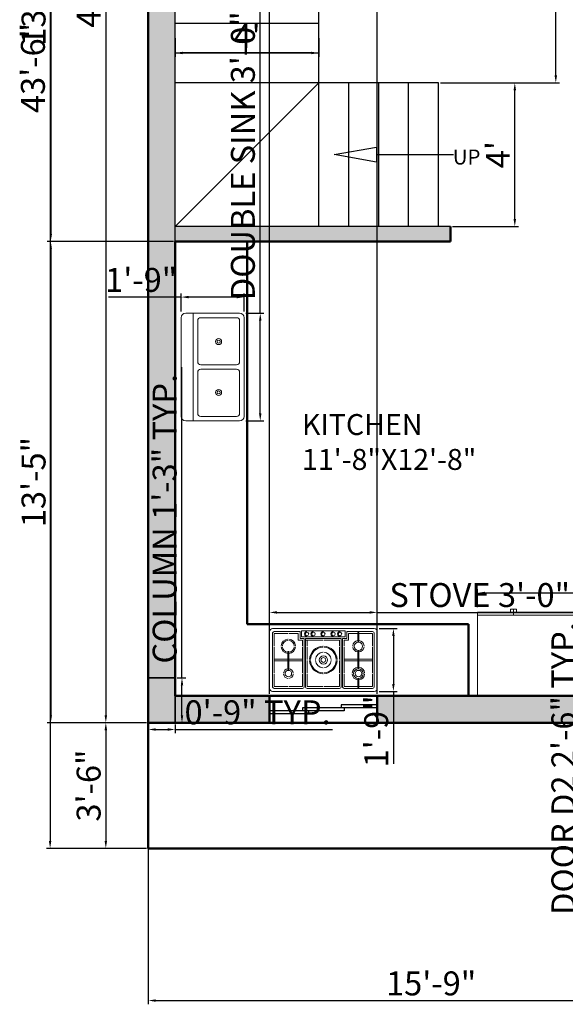
# Model space of a CAD drawing. Units: inches. Extents: x 1770 to 3141, y 984 to 1614.
# Tile 1 of 12: x 1770 to 1952, y 991 to 1320. Entities that reach past the tile are written whole.
import ezdxf

# ---------------------------------------------------------------- set-up
doc = ezdxf.new("R2010")
doc.units = ezdxf.units.IN
for name, color, linetype, lineweight in [('A-ANNO-DIMS', 2, 'Continuous', 18), ('A-ANNO-TEXT', 7, 'Continuous', 18), ('A-AREA-IDEN', 3, 'Continuous', 18), ('A-COLS', 1, 'Continuous', 35), ('A-FLOR-FIXT', 8, 'Continuous', 18), ('A-FLOR-STRS', 7, 'Continuous', 25), ('A-GLAZ', 5, 'Continuous', 25), ('A-WALL', 7, 'Continuous', 50), ('A-WALL-PATT', 8, 'Continuous', 13)]:
    doc.layers.add(name, color=color, linetype=linetype, lineweight=lineweight)
doc.styles.get("Standard").update_dxf_attribs({"font": 'arial.ttf'})
doc.dimstyles.new('ISO-25', dxfattribs={"dimtxt": 8, "dimasz": 2.5, "dimexe": 1.25, "dimexo": 0.625, "dimtad": 1, "dimdec": 1, "dimlunit": 3, "dimtxsty": 'Standard', "dimcen": 2.5, "dimclrt": 1, "dimadec": 0, "dimazin": 0, "dimtfac": 1, "dimtdec": 1, "dimtmove": 0, "dimatfit": 3, "dimfxl": 1, "dimarcsym": 0})

# ---------------------------------------------------------------- blocks, each defined once
blk = doc.blocks.new('STOVE')
for p, q in [((11.85, 19.7), (11.55, 19.7)), ((11.55, 16.92), (11.55, 19.7)), ((11.85, 16.92), (11.55, 16.92)), ((11.85, 16.92), (11.85, 19.7)), ((-11.85, 13.73), (-11.85, 7.62)), ((-11.85, 13.73), (-11.55, 13.73)), ((-11.55, 13.73), (-11.55, 7.62)), ((11.85, 13.23), (11.55, 13.23)), ((11.55, 13.23), (11.55, 7.57)), ((11.85, 13.23), (11.85, 7.57)), ((-11.85, 10.75), (-16.4, 10.75)), ((-11.85, 10.25), (-16.4, 10.25)), ((-7, 10.75), (-11.55, 10.75)), ((-7, 10.25), (-11.55, 10.25)), ((7, 10.75), (11.55, 10.75)), ((7, 10.25), (11.55, 10.25)), ((11.85, 10.75), (16.4, 10.75)), ((11.85, 10.25), (16.4, 10.25)), ((-11.85, 7.62), (-11.55, 7.62)), ((11.85, 7.57), (11.55, 7.57)), ((-7, 3.9), (-8.4, 3.9)), ((-7.8, 3.3), (-7.8, 1)), ((-6.4, 3.3), (-7.8, 3.3)), ((-5.4, 3.9), (-6, 3.9)), ((-5.4, 3.9), (-0.15, 3.9)), ((0.15, 3.9), (5.4, 3.9)), ((6.4, 3.3), (7.8, 3.3)), ((7, 3.9), (8.4, 3.9)), ((7.8, 3.3), (7.8, 1)), ((8.4, 3.9), (8.4, 1.6)), ((11.85, 4.28), (11.55, 4.28)), ((11.55, 4.28), (11.55, 1.3)), ((11.85, 4.28), (11.85, 1.3)), ((7.3, 2.8), (-7.3, 2.8)), ((-7.3, 2.8), (-7.3, 0.8)), ((7.3, 0.8), (-7.3, 0.8)), ((7.3, 2.8), (7.3, 0.8)), ((11.85, 1.3), (11.55, 1.3))]:
    blk.add_line(p, q)
for points in [[(-17, 21), (17, 21, -0.414214), (18, 20), (18, 1, -0.414214), (17, 0), (-17, 0, -0.414214), (-18, 1), (-18, 20, -0.414214)], [(6, 3.3), (-6, 3.3), (-6, 19.4, -0.414214), (-5.4, 20), (5.4, 20, -0.414214), (6, 19.4)]]:
    blk.add_lwpolyline(points, format="xyb", close=True)
for points in [[(-7.8, 1), (-16.4, 1, -0.414214), (-17, 1.6), (-17, 19.4, -0.414214), (-16.4, 20), (-7, 20, -0.414214), (-6.4, 19.4), (-6.4, 3.3)], [(6.4, 19.4, -0.414214), (7, 20), (16.4, 20, -0.414214), (17, 19.4), (17, 1.6, -0.414214), (16.4, 1), (7.8, 1)]]:
    blk.add_lwpolyline(points, format="xyb")
for points in [[(-16.4, 15.22), (-16.4, 19.4), (-11.85, 19.4)], [(-11.55, 19.4), (-7, 19.4), (-7, 15.22)], [(-5.4, 15.22), (-5.4, 19.4), (-0.15, 19.4)], [(0.15, 19.4), (5.4, 19.4), (5.4, 15.22)], [(6.4, 3.3), (6.4, 19.4)], [(7, 15.22), (7, 19.4), (11.55, 19.4)], [(11.85, 19.4), (16.4, 19.4), (16.4, 15.22)], [(-16.4, 6.08), (-16.4, 14.92)], [(-7, 14.92), (-7, 6.08)], [(-5.4, 10.65), (-5.4, 14.92)], [(5.4, 14.92), (5.4, 10.65)], [(7, 6.08), (7, 14.92)], [(16.4, 14.92), (16.4, 6.08)], [(-5.4, 6.08), (-5.4, 10.35)], [(5.4, 10.35), (5.4, 6.08)], [(-11.85, 1.6), (-16.4, 1.6), (-16.4, 5.77)], [(-8.4, 3.9), (-8.4, 1.6), (-11.55, 1.6)], [(-7, 5.77), (-7, 3.9)], [(-5.4, 3.9), (-5.4, 5.77)], [(5.4, 5.77), (5.4, 3.9)], [(7, 3.9), (7, 5.77)], [(16.4, 5.77), (16.4, 1.6), (11.85, 1.6)], [(11.55, 1.6), (8.4, 1.6)]]:
    blk.add_lwpolyline(points)
for centre, radius in [((11.7, 15.07), 1.6), ((-11.7, 15.07), 1.1), ((11.7, 15.07), 1.1), ((0, 10.5), 1.4), ((0, 10.5), 0.8), ((11.7, 5.93), 1.4), ((-5.49, 1.8), 0.6), ((-3.3, 1.8), 0.6), ((0, 1.8), 0.6), ((3.39, 1.8), 0.6), ((5.57, 1.8), 0.6)]:
    blk.add_circle(centre, radius)
for centre, radius, start, end in [((-11.7, 15.07), 1.6, 95.3794, 174.6206), ((-11.7, 15.07), 1.6, 5.3794, 84.6206), ((11.7, 15.07), 2.1, 94.096, 175.904), ((11.7, 15.07), 2.1, 4.096, 85.904), ((-11.7, 15.07), 1.6, 185.3794, 264.6206), ((-11.7, 15.07), 1.6, 275.3794, 354.6206), ((0, 10.5), 4.6, 91.8687, 178.1313), ((0, 10.5), 4.3, 91.9991, 178.0009), ((0, 10.5), 4.6, 1.8687, 88.1313), ((0, 10.5), 4.3, 1.9991, 88.0009), ((11.7, 15.07), 2.1, 184.096, 265.904), ((11.7, 15.07), 2.1, 274.096, 355.904), ((0, 10.5), 4.6, 181.8687, 268.1313), ((0, 10.5), 4.3, 181.9991, 268.0009), ((0, 10.5), 2.6, 93.3074, 176.6926), ((0, 10.5), 2.6, 183.3074, 266.6926), ((0, 10.5), 2.6, 3.3074, 86.6926), ((0, 10.5), 4.6, 271.8687, 358.1313), ((0, 10.5), 4.3, 271.9991, 358.0009), ((0, 10.5), 2.6, 273.3074, 356.6926), ((-11.7, 5.93), 2.4, 93.5833, 176.4167), ((-11.7, 5.93), 2, 94.3012, 175.6988), ((-11.7, 5.93), 2.4, 3.5833, 86.4167), ((-11.7, 5.93), 2, 4.3012, 85.6988), ((11.7, 5.93), 1.9, 94.5281, 175.4719), ((11.7, 5.93), 1.9, 4.5281, 85.4719), ((-11.7, 5.93), 2.4, 183.5833, 266.4167), ((-11.7, 5.93), 2, 184.3012, 265.6988), ((-11.7, 5.93), 2.4, 273.5833, 356.4167), ((-11.7, 5.93), 2, 274.3012, 355.6988), ((11.7, 5.93), 1.9, 184.5281, 265.4719), ((11.7, 5.93), 1.9, 274.5281, 355.4719), ((-5.49, 1.8), 0.846, 89.9979, 270), ((-3.3, 1.8), 0.846, 89.9979, 270), ((0, 1.8), 0.846, 89.9979, 270), ((3.39, 1.8), 0.846, 89.9979, 270), ((5.57, 1.8), 0.846, 89.9979, 270)]:
    blk.add_arc(centre, radius, start, end)
blk = doc.blocks.new('Sink-double - 36 in top')
for p, q in [((-18, -4), (18, -4)), ((-0.75, -18.5), (-0.75, -6.5)), ((0.75, -6.5), (0.75, -18.5))]:
    blk.add_line(p, q)
for points in [[(-16.5, 0), (16.5, 0)], [(-18, -19.5), (-18, -1.5)], [(18, -1.5), (18, -19.5)], [(-16.5, -18.5), (-16.5, -6.5)], [(-15.5, -5.5), (-1.75, -5.5)], [(1.75, -5.5), (15.5, -5.5)], [(16.5, -6.5), (16.5, -18.5)], [(-1.75, -19.5), (-15.5, -19.5)], [(15.5, -19.5), (1.75, -19.5)], [(16.5, -21), (-16.5, -21)]]:
    blk.add_lwpolyline(points)
for centre, radius in [((-8.5, -12.5), 1), ((-8.5, -12.5), 0.5), ((8.5, -12.5), 1), ((8.5, -12.5), 0.5)]:
    blk.add_circle(centre, radius)
for centre, radius, start, end in [((-16.5, -1.5), 1.5, 90, 180), ((16.5, -1.5), 1.5, 0, 90), ((-15.5, -6.5), 1, 90, 180), ((-1.75, -6.5), 1, 0, 90), ((1.75, -6.5), 1, 90, 180), ((15.5, -6.5), 1, 0, 90), ((-16.5, -19.5), 1.5, 180, 270), ((-15.5, -18.5), 1, 180, 270), ((-1.75, -18.5), 1, 270, 0), ((1.75, -18.5), 1, 180, 270), ((15.5, -18.5), 1, 270, 0), ((16.5, -19.5), 1.5, 270, 0)]:
    blk.add_arc(centre, radius, start, end)
blk = doc.blocks.new('Refrigerator-2 door - 36 in top')
for p, q in [((0, -26.999999), (36, -26.999999)), ((11, -27.999999), (11, -28.999999)), ((11, -28.999999), (13, -28.999999)), ((12, -26.999999), (12, -28.999999)), ((13, -28.999999), (13, -27.999999))]:
    blk.add_line(p, q)
blk.add_lwpolyline([(0, -27.999999), (0, 0), (36, 0), (36, -27.999999)], close=True)
blk = doc.blocks.new('*D18')
at = {"layer": 'A-ANNO-DIMS', "color": 0, "lineweight": -2, "transparency": 16777216}
for p, q in [((1812.11, 1565.18), (1797.29, 1565.18)), ((1798.54, 1562.68), (1798.54, 1087.68)), ((1812.11, 1085.18), (1797.29, 1085.18))]:
    blk.add_line(p, q, dxfattribs=at)
at = {"layer": 'A-ANNO-DIMS', "color": 0, "transparency": 16777216}
for points in [[(1798.12, 1562.68), (1798.96, 1562.68), (1798.54, 1565.18)], [(1798.12, 1087.68), (1798.96, 1087.68), (1798.54, 1085.18)]]:
    blk.add_solid(points, dxfattribs=at)
at = {"layer": 'Defpoints', "color": 0, "transparency": 16777216}
for p in [(1812.73, 1565.18), (1798.54, 1085.18), (1812.73, 1085.18)]:
    blk.add_point(p, dxfattribs=at)
at = {"layer": 'A-ANNO-DIMS', "color": 0, "transparency": 16777216, "insert": (1793.83, 1325.18), "char_height": 8, "attachment_point": 5, "rotation": 90}
blk.add_mtext("40'", dxfattribs=at)
blk = doc.blocks.new('*D21')
at = {"layer": 'A-ANNO-DIMS', "color": 0, "lineweight": -2, "transparency": 16777216}
for p, q in [((1812.11, 1085.18), (1797.29, 1085.18)), ((1798.54, 1082.68), (1798.54, 1045.68)), ((1812.11, 1043.18), (1797.29, 1043.18))]:
    blk.add_line(p, q, dxfattribs=at)
at = {"layer": 'A-ANNO-DIMS', "color": 0, "transparency": 16777216}
for points in [[(1798.12, 1082.68), (1798.96, 1082.68), (1798.54, 1085.18)], [(1798.12, 1045.68), (1798.96, 1045.68), (1798.54, 1043.18)]]:
    blk.add_solid(points, dxfattribs=at)
at = {"layer": 'Defpoints', "color": 0, "transparency": 16777216}
for p in [(1812.73, 1085.18), (1798.54, 1043.18), (1812.73, 1043.18)]:
    blk.add_point(p, dxfattribs=at)
at = {"layer": 'A-ANNO-DIMS', "color": 0, "transparency": 16777216, "insert": (1793.83, 1064.18), "char_height": 8, "attachment_point": 5, "rotation": 90}
blk.add_mtext('3\'-6"', dxfattribs=at)
blk = doc.blocks.new('*D59')
at = {"layer": 'A-ANNO-DIMS', "color": 0, "lineweight": -2, "transparency": 16777216}
for p, q in [((1821.73, 1314.13), (1821.73, 1307.93)), ((1869.73, 1314.13), (1869.73, 1307.93)), ((1867.23, 1309.18), (1824.23, 1309.18))]:
    blk.add_line(p, q, dxfattribs=at)
at = {"layer": 'A-ANNO-DIMS', "color": 0, "transparency": 16777216}
for points in [[(1824.23, 1309.6), (1824.23, 1308.76), (1821.73, 1309.18)], [(1867.23, 1309.6), (1867.23, 1308.76), (1869.73, 1309.18)]]:
    blk.add_solid(points, dxfattribs=at)
at = {"layer": 'Defpoints', "color": 0, "transparency": 16777216}
for p in [(1821.73, 1314.76), (1869.73, 1314.76), (1821.73, 1309.18)]:
    blk.add_point(p, dxfattribs=at)
at = {"layer": 'A-ANNO-DIMS', "color": 0, "transparency": 16777216, "insert": (1845.73, 1313.8), "char_height": 8, "attachment_point": 5}
blk.add_mtext("4'", dxfattribs=at)
blk = doc.blocks.new('*D61')
at = {"layer": 'A-ANNO-DIMS', "color": 0, "lineweight": -2, "transparency": 16777216}
for p, q in [((1910.36, 1407.18), (1950.15, 1407.18)), ((1948.9, 1301.68), (1948.9, 1404.68)), ((1910.36, 1299.18), (1950.15, 1299.18))]:
    blk.add_line(p, q, dxfattribs=at)
at = {"layer": 'A-ANNO-DIMS', "color": 0, "transparency": 16777216}
for points in [[(1948.49, 1404.68), (1949.32, 1404.68), (1948.9, 1407.18)], [(1948.49, 1301.68), (1949.32, 1301.68), (1948.9, 1299.18)]]:
    blk.add_solid(points, dxfattribs=at)
at = {"layer": 'Defpoints', "color": 0, "transparency": 16777216}
for p in [(1909.73, 1407.18), (1948.9, 1407.18), (1909.73, 1299.18)]:
    blk.add_point(p, dxfattribs=at)
at = {"layer": 'A-ANNO-DIMS', "color": 0, "transparency": 16777216, "insert": (1944.19, 1353.18), "char_height": 8, "attachment_point": 5, "rotation": 90}
blk.add_mtext("9'", dxfattribs=at)
blk = doc.blocks.new('*D62')
at = {"layer": 'A-ANNO-DIMS', "color": 0, "lineweight": -2, "transparency": 16777216}
for p, q in [((1910.36, 1299.18), (1936.45, 1299.18)), ((1935.2, 1253.68), (1935.2, 1296.68)), ((1914.36, 1251.18), (1936.45, 1251.18))]:
    blk.add_line(p, q, dxfattribs=at)
at = {"layer": 'A-ANNO-DIMS', "color": 0, "transparency": 16777216}
for points in [[(1934.78, 1296.68), (1935.61, 1296.68), (1935.2, 1299.18)], [(1934.78, 1253.68), (1935.61, 1253.68), (1935.2, 1251.18)]]:
    blk.add_solid(points, dxfattribs=at)
at = {"layer": 'Defpoints', "color": 0, "transparency": 16777216}
for p in [(1909.73, 1299.18), (1935.2, 1299.18), (1913.73, 1251.18)]:
    blk.add_point(p, dxfattribs=at)
at = {"layer": 'A-ANNO-DIMS', "color": 0, "transparency": 16777216, "insert": (1930.57, 1275.18), "char_height": 8, "attachment_point": 5, "rotation": 90}
blk.add_mtext("4'", dxfattribs=at)
blk = doc.blocks.new('*D65')
at = {"layer": 'A-ANNO-DIMS', "color": 0, "lineweight": -2, "transparency": 16777216}
for p, q in [((1812.11, 1565.18), (1778.67, 1565.18)), ((1779.92, 1562.68), (1779.92, 1045.68)), ((1812.11, 1043.18), (1778.67, 1043.18))]:
    blk.add_line(p, q, dxfattribs=at)
at = {"layer": 'A-ANNO-DIMS', "color": 0, "transparency": 16777216}
for points in [[(1779.51, 1562.68), (1780.34, 1562.68), (1779.92, 1565.18)], [(1779.51, 1045.68), (1780.34, 1045.68), (1779.92, 1043.18)]]:
    blk.add_solid(points, dxfattribs=at)
at = {"layer": 'Defpoints', "color": 0, "transparency": 16777216}
for p in [(1812.73, 1565.18), (1779.92, 1043.18), (1812.73, 1043.18)]:
    blk.add_point(p, dxfattribs=at)
at = {"layer": 'A-ANNO-DIMS', "color": 0, "transparency": 16777216, "insert": (1775.21, 1304.18), "char_height": 8, "attachment_point": 5, "rotation": 90}
blk.add_mtext('43\'-6"', dxfattribs=at)
blk = doc.blocks.new('COLUMN-9x15')
at = {"transparency": 33554687}
h = blk.add_hatch(color=256, dxfattribs=at)
h.dxf.hatch_style = 1
h.paths.add_polyline_path([(9, 15), (0, 15), (0, 0), (9, 0)])
blk.add_lwpolyline([(9, 15), (0, 15), (0, 0), (9, 0)], close=True)
blk = doc.blocks.new('*D68')
at = {"layer": 'A-ANNO-DIMS', "color": 0, "lineweight": -2, "transparency": 16777216}
for p, q in [((1823.98, 1100.18), (1823.98, 1204.14)), ((1822.36, 1100.18), (1825.23, 1100.18)), ((1823.98, 1087.68), (1823.98, 1097.68)), ((1822.36, 1085.18), (1825.23, 1085.18))]:
    blk.add_line(p, q, dxfattribs=at)
at = {"layer": 'A-ANNO-DIMS', "color": 0, "transparency": 16777216}
for points in [[(1823.57, 1097.68), (1824.4, 1097.68), (1823.98, 1100.18)], [(1823.57, 1087.68), (1824.4, 1087.68), (1823.98, 1085.18)]]:
    blk.add_solid(points, dxfattribs=at)
at = {"layer": 'Defpoints', "color": 0, "transparency": 16777216}
for p in [(1821.73, 1100.18), (1823.98, 1100.18), (1821.73, 1085.18)]:
    blk.add_point(p, dxfattribs=at)
at = {"layer": 'A-ANNO-DIMS', "color": 1, "transparency": 16777216, "insert": (1819.22, 1153.41), "char_height": 8, "attachment_point": 5, "rotation": 90}
blk.add_mtext('COLUMN 1\'-3" TYP.', dxfattribs=at)
blk = doc.blocks.new('*D69')
at = {"layer": 'A-ANNO-DIMS', "color": 0, "lineweight": -2, "transparency": 16777216}
for p, q in [((1812.73, 1084.55), (1812.73, 1081.68)), ((1821.73, 1084.55), (1821.73, 1081.68)), ((1815.23, 1082.93), (1819.23, 1082.93)), ((1821.73, 1082.93), (1874.25, 1082.93))]:
    blk.add_line(p, q, dxfattribs=at)
at = {"layer": 'A-ANNO-DIMS', "color": 0, "transparency": 16777216}
for points in [[(1815.23, 1083.35), (1815.23, 1082.51), (1812.73, 1082.93)], [(1819.23, 1083.35), (1819.23, 1082.51), (1821.73, 1082.93)]]:
    blk.add_solid(points, dxfattribs=at)
at = {"layer": 'Defpoints', "color": 0, "transparency": 16777216}
for p in [(1812.73, 1085.18), (1821.73, 1085.18), (1821.73, 1082.93)]:
    blk.add_point(p, dxfattribs=at)
at = {"layer": 'A-ANNO-DIMS', "color": 1, "transparency": 16777216, "insert": (1849.24, 1087.64), "char_height": 8, "attachment_point": 5}
blk.add_mtext('0\'-9" TYP.', dxfattribs=at)
blk = doc.blocks.new('*D70')
at = {"layer": 'A-ANNO-DIMS', "color": 0, "lineweight": -2, "transparency": 16777216}
for p, q in [((1961.11, 1154.18), (1955.98, 1154.18)), ((1957.23, 1151.68), (1957.23, 1126.68)), ((1961.11, 1124.18), (1955.98, 1124.18)), ((1957.23, 1124.18), (1957.23, 1018.04))]:
    blk.add_line(p, q, dxfattribs=at)
at = {"layer": 'A-ANNO-DIMS', "color": 0, "transparency": 16777216}
for points in [[(1956.82, 1151.68), (1957.65, 1151.68), (1957.23, 1154.18)], [(1956.82, 1126.68), (1957.65, 1126.68), (1957.23, 1124.18)]]:
    blk.add_solid(points, dxfattribs=at)
at = {"layer": 'Defpoints', "color": 0, "transparency": 16777216}
for p in [(1961.73, 1154.18), (1957.23, 1124.18), (1961.73, 1124.18)]:
    blk.add_point(p, dxfattribs=at)
at = {"layer": 'A-ANNO-DIMS', "color": 1, "transparency": 16777216, "insert": (1952.47, 1069.86), "char_height": 8, "attachment_point": 5, "rotation": 90}
blk.add_mtext('DOOR D2 2\'-6" TYP.', dxfattribs=at)
blk = doc.blocks.new('*D82')
at = {"layer": 'A-ANNO-DIMS', "color": 0, "lineweight": -2, "transparency": 16777216}
for p, q in [((1853.23, 1117.3), (1853.23, 1123.33)), ((1889.23, 1117.3), (1889.23, 1123.33)), ((1855.73, 1122.08), (1886.73, 1122.08)), ((1889.23, 1122.08), (1955.2, 1122.08))]:
    blk.add_line(p, q, dxfattribs=at)
at = {"layer": 'A-ANNO-DIMS', "color": 0, "transparency": 16777216}
for points in [[(1855.73, 1122.5), (1855.73, 1121.66), (1853.23, 1122.08)], [(1886.73, 1122.5), (1886.73, 1121.66), (1889.23, 1122.08)]]:
    blk.add_solid(points, dxfattribs=at)
at = {"layer": 'Defpoints', "color": 0, "transparency": 16777216}
for p in [(1889.23, 1122.08), (1853.23, 1116.68), (1889.23, 1116.68)]:
    blk.add_point(p, dxfattribs=at)
at = {"layer": 'A-ANNO-DIMS', "color": 1, "transparency": 16777216, "insert": (1923.47, 1126.85), "char_height": 8, "attachment_point": 5}
blk.add_mtext('STOVE 3\'-0"', dxfattribs=at)
blk = doc.blocks.new('*D83')
at = {"layer": 'A-ANNO-DIMS', "color": 0, "lineweight": -2, "transparency": 16777216}
for p, q in [((1889.86, 1116.68), (1895.88, 1116.68)), ((1894.63, 1114.18), (1894.63, 1098.18)), ((1889.86, 1095.68), (1895.88, 1095.68)), ((1894.63, 1095.68), (1894.63, 1071.42))]:
    blk.add_line(p, q, dxfattribs=at)
at = {"layer": 'A-ANNO-DIMS', "color": 0, "transparency": 16777216}
for points in [[(1894.22, 1114.18), (1895.05, 1114.18), (1894.63, 1116.68)], [(1894.22, 1098.18), (1895.05, 1098.18), (1894.63, 1095.68)]]:
    blk.add_solid(points, dxfattribs=at)
at = {"layer": 'Defpoints', "color": 0, "transparency": 16777216}
for p in [(1889.23, 1116.68), (1889.23, 1095.68), (1894.63, 1095.68)]:
    blk.add_point(p, dxfattribs=at)
at = {"layer": 'A-ANNO-DIMS', "color": 1, "transparency": 16777216, "insert": (1889.92, 1082.3), "char_height": 8, "attachment_point": 5, "rotation": 90}
blk.add_mtext('1\'-9"', dxfattribs=at)
blk = doc.blocks.new('*D84')
at = {"layer": 'A-ANNO-DIMS', "color": 0, "lineweight": -2, "transparency": 16777216}
for p, q in [((1850.13, 1222.14), (1850.13, 1325.01)), ((1845.36, 1222.14), (1851.38, 1222.14)), ((1850.13, 1188.64), (1850.13, 1219.64)), ((1845.36, 1186.14), (1851.38, 1186.14))]:
    blk.add_line(p, q, dxfattribs=at)
at = {"layer": 'A-ANNO-DIMS', "color": 0, "transparency": 16777216}
for points in [[(1849.72, 1219.64), (1850.55, 1219.64), (1850.13, 1222.14)], [(1849.72, 1188.64), (1850.55, 1188.64), (1850.13, 1186.14)]]:
    blk.add_solid(points, dxfattribs=at)
at = {"layer": 'Defpoints', "color": 0, "transparency": 16777216}
for p in [(1844.73, 1222.14), (1850.13, 1222.14), (1844.73, 1186.14)]:
    blk.add_point(p, dxfattribs=at)
at = {"layer": 'A-ANNO-DIMS', "color": 1, "transparency": 16777216, "insert": (1845.37, 1274.82), "char_height": 8, "attachment_point": 5, "rotation": 90}
blk.add_mtext('DOUBLE SINK 3\'-0"', dxfattribs=at)
blk = doc.blocks.new('*D85')
at = {"layer": 'A-ANNO-DIMS', "color": 0, "lineweight": -2, "transparency": 16777216}
for p, q in [((1823.73, 1222.76), (1823.73, 1228.79)), ((1844.73, 1222.76), (1844.73, 1228.79)), ((1823.73, 1227.54), (1799.47, 1227.54)), ((1842.23, 1227.54), (1826.23, 1227.54))]:
    blk.add_line(p, q, dxfattribs=at)
at = {"layer": 'A-ANNO-DIMS', "color": 0, "transparency": 16777216}
for points in [[(1826.23, 1227.96), (1826.23, 1227.12), (1823.73, 1227.54)], [(1842.23, 1227.96), (1842.23, 1227.12), (1844.73, 1227.54)]]:
    blk.add_solid(points, dxfattribs=at)
at = {"layer": 'Defpoints', "color": 0, "transparency": 16777216}
for p in [(1823.73, 1227.54), (1823.73, 1222.14), (1844.73, 1222.14)]:
    blk.add_point(p, dxfattribs=at)
at = {"layer": 'A-ANNO-DIMS', "color": 1, "transparency": 16777216, "insert": (1810.35, 1232.25), "char_height": 8, "attachment_point": 5}
blk.add_mtext('1\'-9"', dxfattribs=at)
blk = doc.blocks.new('*D86')
at = {"layer": 'A-ANNO-DIMS', "color": 0, "lineweight": -2, "transparency": 16777216}
for p, q in [((1922.74, 1123.8), (1922.74, 1129.83)), ((1958.74, 1123.8), (1958.74, 1129.83)), ((1925.24, 1128.58), (1956.24, 1128.58)), ((1958.74, 1128.58), (2075.24, 1128.58))]:
    blk.add_line(p, q, dxfattribs=at)
at = {"layer": 'A-ANNO-DIMS', "color": 0, "transparency": 16777216}
for points in [[(1925.24, 1129), (1925.24, 1128.16), (1922.74, 1128.58)], [(1956.24, 1129), (1956.24, 1128.16), (1958.74, 1128.58)]]:
    blk.add_solid(points, dxfattribs=at)
at = {"layer": 'Defpoints', "color": 0, "transparency": 16777216}
for p in [(1958.74, 1128.58), (1922.74, 1123.18), (1958.74, 1123.18)]:
    blk.add_point(p, dxfattribs=at)
at = {"layer": 'A-ANNO-DIMS', "color": 1, "transparency": 16777216, "insert": (2018.24, 1133.35), "char_height": 8, "attachment_point": 5}
blk.add_mtext('REFRIGERATOR 3\'-0"', dxfattribs=at)
blk = doc.blocks.new('*D108')
at = {"layer": 'A-ANNO-DIMS', "color": 0, "lineweight": -2, "transparency": 16777216}
for p, q in [((1821.11, 1407.18), (1778.88, 1407.18)), ((1780.13, 1404.68), (1780.13, 1248.68)), ((1821.11, 1246.18), (1778.88, 1246.18))]:
    blk.add_line(p, q, dxfattribs=at)
at = {"layer": 'A-ANNO-DIMS', "color": 0, "transparency": 16777216}
for points in [[(1779.72, 1404.68), (1780.55, 1404.68), (1780.13, 1407.18)], [(1779.72, 1248.68), (1780.55, 1248.68), (1780.13, 1246.18)]]:
    blk.add_solid(points, dxfattribs=at)
at = {"layer": 'Defpoints', "color": 0, "transparency": 16777216}
for p in [(1821.73, 1407.18), (1780.13, 1246.18), (1821.73, 1246.18)]:
    blk.add_point(p, dxfattribs=at)
at = {"layer": 'A-ANNO-DIMS', "color": 1, "transparency": 16777216, "insert": (1775.42, 1326.68), "char_height": 8, "attachment_point": 5, "rotation": 90}
blk.add_mtext('13\'-5"', dxfattribs=at)
blk = doc.blocks.new('*D109')
at = {"layer": 'A-ANNO-DIMS', "color": 0, "lineweight": -2, "transparency": 16777216}
for p, q in [((1821.11, 1246.18), (1778.88, 1246.18)), ((1780.13, 1243.68), (1780.13, 1087.68)), ((1812.11, 1085.18), (1778.88, 1085.18))]:
    blk.add_line(p, q, dxfattribs=at)
at = {"layer": 'A-ANNO-DIMS', "color": 0, "transparency": 16777216}
for points in [[(1779.72, 1243.68), (1780.55, 1243.68), (1780.13, 1246.18)], [(1779.72, 1087.68), (1780.55, 1087.68), (1780.13, 1085.18)]]:
    blk.add_solid(points, dxfattribs=at)
at = {"layer": 'Defpoints', "color": 0, "transparency": 16777216}
for p in [(1821.73, 1246.18), (1780.13, 1085.18), (1812.73, 1085.18)]:
    blk.add_point(p, dxfattribs=at)
at = {"layer": 'A-ANNO-DIMS', "color": 1, "transparency": 16777216, "insert": (1775.42, 1165.68), "char_height": 8, "attachment_point": 5, "rotation": 90}
blk.add_mtext('13\'-5"', dxfattribs=at)
blk = doc.blocks.new('*D110')
at = {"layer": 'A-ANNO-DIMS', "color": 0, "lineweight": -2, "transparency": 16777216}
for p, q in [((1812.73, 1084.55), (1812.73, 991.02)), ((2001.73, 1084.55), (2001.73, 991.02)), ((1815.23, 992.27), (1999.23, 992.27))]:
    blk.add_line(p, q, dxfattribs=at)
at = {"layer": 'A-ANNO-DIMS', "color": 0, "transparency": 16777216}
for points in [[(1815.23, 992.69), (1815.23, 991.85), (1812.73, 992.27)], [(1999.23, 992.69), (1999.23, 991.85), (2001.73, 992.27)]]:
    blk.add_solid(points, dxfattribs=at)
at = {"layer": 'Defpoints', "color": 0, "transparency": 16777216}
for p in [(1812.73, 1085.18), (2001.73, 1085.18), (2001.73, 992.27)]:
    blk.add_point(p, dxfattribs=at)
at = {"layer": 'A-ANNO-DIMS', "color": 1, "transparency": 16777216, "insert": (1907.23, 996.98), "char_height": 8, "attachment_point": 5}
blk.add_mtext('15\'-9"', dxfattribs=at)
blk = doc.blocks.new('*D114')
at = {"layer": 'A-ANNO-DIMS', "color": 0, "lineweight": -2, "transparency": 16777216}
for p, q in [((1821.73, 1094.8), (1821.73, 1599.03)), ((1824.23, 1597.78), (1850.73, 1597.78)), ((1853.23, 1094.8), (1853.23, 1599.03)), ((1853.23, 1597.78), (1897.03, 1597.78))]:
    blk.add_line(p, q, dxfattribs=at)
at = {"layer": 'A-ANNO-DIMS', "color": 0, "transparency": 16777216}
for points in [[(1824.23, 1598.2), (1824.23, 1597.36), (1821.73, 1597.78)], [(1850.73, 1598.2), (1850.73, 1597.36), (1853.23, 1597.78)]]:
    blk.add_solid(points, dxfattribs=at)
at = {"layer": 'Defpoints', "color": 0, "transparency": 16777216}
for p in [(1853.23, 1597.78), (1821.73, 1094.18), (1853.23, 1094.18)]:
    blk.add_point(p, dxfattribs=at)
at = {"layer": 'A-ANNO-DIMS', "color": 1, "transparency": 16777216, "insert": (1876.38, 1602.54), "char_height": 8, "attachment_point": 5}
blk.add_mtext('2\'-7 1/2"', dxfattribs=at)
blk = doc.blocks.new('*D115')
at = {"layer": 'A-ANNO-DIMS', "color": 0, "lineweight": -2, "transparency": 16777216}
for p, q in [((1853.23, 1094.8), (1853.23, 1599.03)), ((1855.73, 1597.78), (1886.73, 1597.78)), ((1889.23, 1094.8), (1889.23, 1599.03))]:
    blk.add_line(p, q, dxfattribs=at)
at = {"layer": 'A-ANNO-DIMS', "color": 0, "transparency": 16777216}
for points in [[(1855.73, 1598.2), (1855.73, 1597.36), (1853.23, 1597.78)], [(1886.73, 1598.2), (1886.73, 1597.36), (1889.23, 1597.78)]]:
    blk.add_solid(points, dxfattribs=at)
at = {"layer": 'Defpoints', "color": 0, "transparency": 16777216}
for p in [(1889.23, 1597.78), (1853.23, 1094.18), (1889.23, 1094.18)]:
    blk.add_point(p, dxfattribs=at)
at = {"layer": 'A-ANNO-DIMS', "color": 1, "transparency": 16777216, "insert": (1871.23, 1602.49), "char_height": 8, "attachment_point": 5}
blk.add_mtext('3\'-0"', dxfattribs=at)

msp = doc.modelspace()

# ---------------------------------------------------------------- hatches: boundary and pattern name
at = {"layer": 'A-WALL-PATT'}
h = msp.add_hatch(color=256, dxfattribs=at)
h.dxf.hatch_style = 1
h.paths.add_polyline_path([(1821.73, 1556.18), (1844.25, 1556.18), (2086.73, 1556.18), (2086.73, 1443.18), (2091.73, 1443.18), (2091.73, 1556.18), (2239.73, 1556.18), (2239.73, 1565.18), (1812.73, 1565.18), (1812.73, 1100.18), (1821.73, 1100.18), (1821.73, 1246.18), (1913.73, 1246.18), (1913.73, 1251.18), (1821.73, 1251.18), (1821.73, 1407.18), (1944.73, 1407.18), (1944.73, 1412.18), (1821.73, 1412.18)])
h.paths.add_polyline_path([(1985.73, 1515.18), (1997.73, 1515.18), (1997.73, 1520.18), (1980.73, 1520.18), (1980.73, 1478.18), (1985.73, 1478.18)], flags=16)
h.paths.add_polyline_path([(2038.73, 1520.18), (2021.73, 1520.18), (2021.73, 1515.18), (2033.73, 1515.18), (2033.73, 1412.18), (1985.73, 1412.18), (1985.73, 1448.18), (1980.73, 1448.18), (1980.73, 1407.18), (2038.73, 1407.18), (2038.73, 1443.18), (2056.73, 1443.18), (2056.73, 1448.18), (2038.73, 1448.18)], flags=17)
h.paths.add_polyline_path([(1853.23, 1094.18), (1821.73, 1094.18), (1821.73, 1085.18), (1853.23, 1085.18)])
h.paths.add_polyline_path([(2001.73, 1094.18), (1966.73, 1094.18), (1966.73, 1124.18), (1961.73, 1124.18), (1961.73, 1094.18), (1889.23, 1094.18), (1889.23, 1085.18), (2001.73, 1085.18)])
h.paths.add_polyline_path([(2020.69, 1094.18), (2010.73, 1094.18), (2010.73, 1085.18), (2020.69, 1085.18)])
h.paths.add_polyline_path([(2116.73, 1094.18), (2080.69, 1094.18), (2080.69, 1085.18), (2116.73, 1085.18)])
h.paths.add_polyline_path([(2125.73, 1184.68), (2116.73, 1184.68), (2116.73, 1159.18), (2056.73, 1159.18), (2056.73, 1246.18), (2086.73, 1246.18), (2086.73, 1251.18), (2001.73, 1251.18), (2001.73, 1246.18), (2051.73, 1246.18), (2051.73, 1159.18), (1966.73, 1159.18), (1966.73, 1246.18), (1971.73, 1246.18), (1971.73, 1251.18), (1961.73, 1251.18), (1961.73, 1154.18), (1991.73, 1154.18), (2125.73, 1154.18)], flags=17)
h.paths.add_polyline_path([(2125.73, 1256.18), (2116.73, 1256.18), (2116.73, 1220.68), (2125.73, 1220.68)], flags=17)
h.paths.add_polyline_path([(2128.73, 1309.18), (2116.73, 1309.18), (2116.73, 1292.18), (2125.73, 1292.18), (2125.73, 1300.18), (2128.73, 1300.18)], flags=17)
h.paths.add_polyline_path([(2239.73, 1309.18), (2217.73, 1309.18), (2217.73, 1300.18), (2239.73, 1300.18)], flags=17)
h.paths.add_polyline_path([(2181.73, 1309.18), (2176.73, 1309.18), (2176.73, 1300.18), (2181.73, 1300.18)], flags=17)

# ---------------------------------------------------------------- linework, layer by layer
at = {"layer": 'A-FLOR-STRS'}
for p, q in [((1821.73, 1251.18), (1821.73, 1407.18)), ((1869.73, 1251.18), (1869.73, 1407.18)), ((1821.73, 1319.18), (1869.73, 1319.18)), ((1821.73, 1309.18), (1869.73, 1309.18)), ((1909.73, 1299.18), (1821.73, 1299.18)), ((1869.73, 1299.18), (1821.73, 1251.18)), ((1879.73, 1251.18), (1879.73, 1299.18)), ((1889.73, 1251.18), (1889.73, 1299.18)), ((1899.73, 1251.18), (1899.73, 1299.18)), ((1909.73, 1251.18), (1909.73, 1299.18)), ((1888.98, 1275.18), (1914.71, 1275.18)), ((1913.73, 1251.18), (1821.73, 1251.18))]:
    msp.add_line(p, q, dxfattribs=at)
msp.add_lwpolyline([(1874.82, 1275.18), (1888.98, 1277.73), (1888.98, 1272.63)], close=True, dxfattribs=at)
at = {"layer": 'A-GLAZ'}
for p, q in [((1889.23, 1090.18), (1864.23, 1090.18)), ((1864.23, 1090.18), (1864.23, 1089.18)), ((1877.23, 1091.18), (1877.23, 1090.18)), ((1889.23, 1091.18), (1877.23, 1091.18)), ((1878.23, 1090.18), (1878.23, 1089.18)), ((1878.23, 1089.18), (1853.23, 1089.18)), ((1866.23, 1088.18), (1853.23, 1088.18)), ((1866.23, 1089.18), (1866.23, 1088.18))]:
    msp.add_line(p, q, dxfattribs=at)
at = {"layer": 'A-WALL'}
for p, q in [((1812.73, 1043.18), (1812.73, 1565.18)), ((1913.73, 1246.18), (1913.73, 1251.18)), ((1821.73, 1094.18), (1821.73, 1246.18)), ((1913.73, 1246.18), (1821.73, 1246.18)), ((1845.73, 1118.18), (1845.73, 1246.18)), ((1919.73, 1118.18), (1845.73, 1118.18)), ((1919.73, 1094.18), (1919.73, 1118.18)), ((1961.73, 1094.18), (1821.73, 1094.18)), ((1853.23, 1094.18), (1853.23, 1085.18)), ((1889.23, 1094.18), (1889.23, 1085.18)), ((2412.73, 1085.18), (1812.73, 1085.18)), ((2412.73, 1043.18), (1812.73, 1043.18))]:
    msp.add_line(p, q, dxfattribs=at)

# ---------------------------------------------------------------- block references
at = {"layer": 'A-COLS'}
msp.add_blockref('COLUMN-9x15', (1812.73, 1085.18), dxfattribs=at)
at = {"layer": 'A-FLOR-FIXT', "rotation": 90}
msp.add_blockref('Sink-double - 36 in top', (1823.73, 1204.14), dxfattribs=at)
at = {"layer": 'A-FLOR-FIXT', "xscale": -1, "rotation": 180}
for name, p in [('Refrigerator-2 door - 36 in top', (1922.74, 1094.18)), ('STOVE', (1871.23, 1116.68))]:
    msp.add_blockref(name, p, dxfattribs=at)

# ---------------------------------------------------------------- texts
at = {"layer": 'A-ANNO-TEXT', "insert": (1923.71, 1276.88), "char_height": 5, "attachment_point": 3}
msp.add_mtext_dynamic_manual_height_columns('UP', width=10.7355, gutter_width=12.5, heights=[0], dxfattribs=at)
at = {"layer": 'A-AREA-IDEN', "insert": (1864.08, 1188.41), "char_height": 7, "attachment_point": 1}
msp.add_mtext_dynamic_manual_height_columns('KITCHEN\\P11\'-8"X12\'-8"', width=86.9528, gutter_width=12.5, heights=[0], dxfattribs=at)

# ---------------------------------------------------------------- dimensions: what is measured, and where the dimension line sits
at = {"layer": 'A-ANNO-DIMS'}
for base, p1, p2, override, picture, middle in [((1853.23, 1597.78), (1821.73, 1094.18), (1853.23, 1094.18), {"dimdec": 1, "dimlfac": 1, "dimrnd": 0, "dimzin": 1, "dimdsep": 46, "dimlunit": 4, "dimfrac": 2}, '*D114', (1876.38, 1602.54)), ((1889.23, 1597.78), (1853.23, 1094.18), (1889.23, 1094.18), {"dimdec": 1, "dimlfac": 1, "dimrnd": 0, "dimzin": 1, "dimdsep": 46, "dimlunit": 4, "dimfrac": 2}, '*D115', (1871.23, 1602.49)), ((1821.73, 1309.18), (1869.73, 1314.76), (1821.73, 1314.76), {"dimclrd": 0, "dimclre": 0, "dimclrt": 0}, '*D59', (1845.73, 1313.8)), ((2001.73, 992.27), (1812.73, 1085.18), (2001.73, 1085.18), {"dimdec": 1, "dimlfac": 1, "dimrnd": 0, "dimzin": 1, "dimdsep": 46, "dimlunit": 4, "dimfrac": 2}, '*D110', (1907.23, 996.98))]:
    dim = msp.add_linear_dim(base=base, p1=p1, p2=p2, dimstyle='ISO-25', override=override, dxfattribs=at)
    dim.commit()
    dim.dimension.update_dxf_attribs({"geometry": picture, "text_midpoint": middle})
for base, p1, p2, angle, override, picture, middle in [((1779.92, 1043.18), (1812.73, 1565.18), (1812.73, 1043.18), 90, {"dimclrd": 0, "dimclre": 0, "dimclrt": 0}, '*D65', (1775.21, 1304.18)), ((1798.54, 1085.18), (1812.73, 1565.18), (1812.73, 1085.18), 90, {"dimclrd": 0, "dimclre": 0, "dimclrt": 0}, '*D18', (1793.83, 1325.18)), ((1780.13, 1246.18), (1821.73, 1407.18), (1821.73, 1246.18), 90, {"dimdec": 1, "dimlfac": 1, "dimrnd": 0, "dimzin": 1, "dimdsep": 46, "dimlunit": 4, "dimfrac": 2}, '*D108', (1775.42, 1326.68)), ((1948.9, 1407.18), (1909.73, 1299.18), (1909.73, 1407.18), 90, {"dimclrd": 0, "dimclre": 0, "dimclrt": 0}, '*D61', (1944.19, 1353.18)), ((1935.2, 1299.18), (1913.73, 1251.18), (1909.73, 1299.18), 90, {"dimclrd": 0, "dimclre": 0, "dimclrt": 0}, '*D62', (1930.57, 1275.18)), ((1780.13, 1085.18), (1821.73, 1246.18), (1812.73, 1085.18), 90, {"dimdec": 1, "dimlfac": 1, "dimrnd": 0, "dimzin": 1, "dimdsep": 46, "dimlunit": 4, "dimfrac": 2}, '*D109', (1775.42, 1165.68)), ((1823.73, 1227.54), (1844.73, 1222.14), (1823.73, 1222.14), 180, {"dimdec": 1, "dimrnd": 0, "dimzin": 1, "dimlunit": 4, "dimfrac": 2}, '*D85', (1810.35, 1232.25)), ((1894.63, 1095.68), (1889.23, 1116.68), (1889.23, 1095.68), 270, {"dimdec": 1, "dimrnd": 0, "dimzin": 1, "dimlunit": 4, "dimfrac": 2}, '*D83', (1889.92, 1082.3)), ((1798.54, 1043.18), (1812.73, 1085.18), (1812.73, 1043.18), 90, {"dimclrd": 0, "dimclre": 0, "dimclrt": 0}, '*D21', (1793.83, 1064.18))]:
    dim = msp.add_linear_dim(base=base, p1=p1, p2=p2, angle=angle, dimstyle='ISO-25', override=override, dxfattribs=at)
    dim.commit()
    dim.dimension.update_dxf_attribs({"geometry": picture, "text_midpoint": middle})
for base, p1, p2, angle, text, picture, middle in [((1850.13, 1222.14), (1844.73, 1186.14), (1844.73, 1222.14), 90, 'DOUBLE SINK <>', '*D84', (1845.37, 1274.82)), ((1823.98, 1100.18), (1821.73, 1085.18), (1821.73, 1100.18), 90, 'COLUMN <> TYP.', '*D68', (1819.22, 1153.41)), ((1957.23, 1124.18), (1961.73, 1154.18), (1961.73, 1124.18), 270, 'DOOR D2 <> TYP.', '*D70', (1952.47, 1069.86))]:
    dim = msp.add_linear_dim(base=base, p1=p1, p2=p2, angle=angle, text=text, dimstyle='ISO-25', override={"dimdec": 1, "dimrnd": 0, "dimzin": 1, "dimlunit": 4, "dimfrac": 2}, dxfattribs=at)
    dim.commit()
    dim.dimension.update_dxf_attribs({"geometry": picture, "text_midpoint": middle})
for base, p1, p2, text, picture, middle in [((1958.74, 1128.58), (1922.74, 1123.18), (1958.74, 1123.18), 'REFRIGERATOR <>', '*D86', (2018.24, 1133.35)), ((1889.23, 1122.08), (1853.23, 1116.68), (1889.23, 1116.68), 'STOVE <>', '*D82', (1923.47, 1126.85)), ((1821.73, 1082.93), (1812.73, 1085.18), (1821.73, 1085.18), '<> TYP.', '*D69', (1849.24, 1087.64))]:
    dim = msp.add_linear_dim(base=base, p1=p1, p2=p2, text=text, dimstyle='ISO-25', override={"dimdec": 1, "dimrnd": 0, "dimzin": 1, "dimlunit": 4, "dimfrac": 2}, dxfattribs=at)
    dim.commit()
    dim.dimension.update_dxf_attribs({"geometry": picture, "text_midpoint": middle})

doc.saveas('drawing.dxf')
